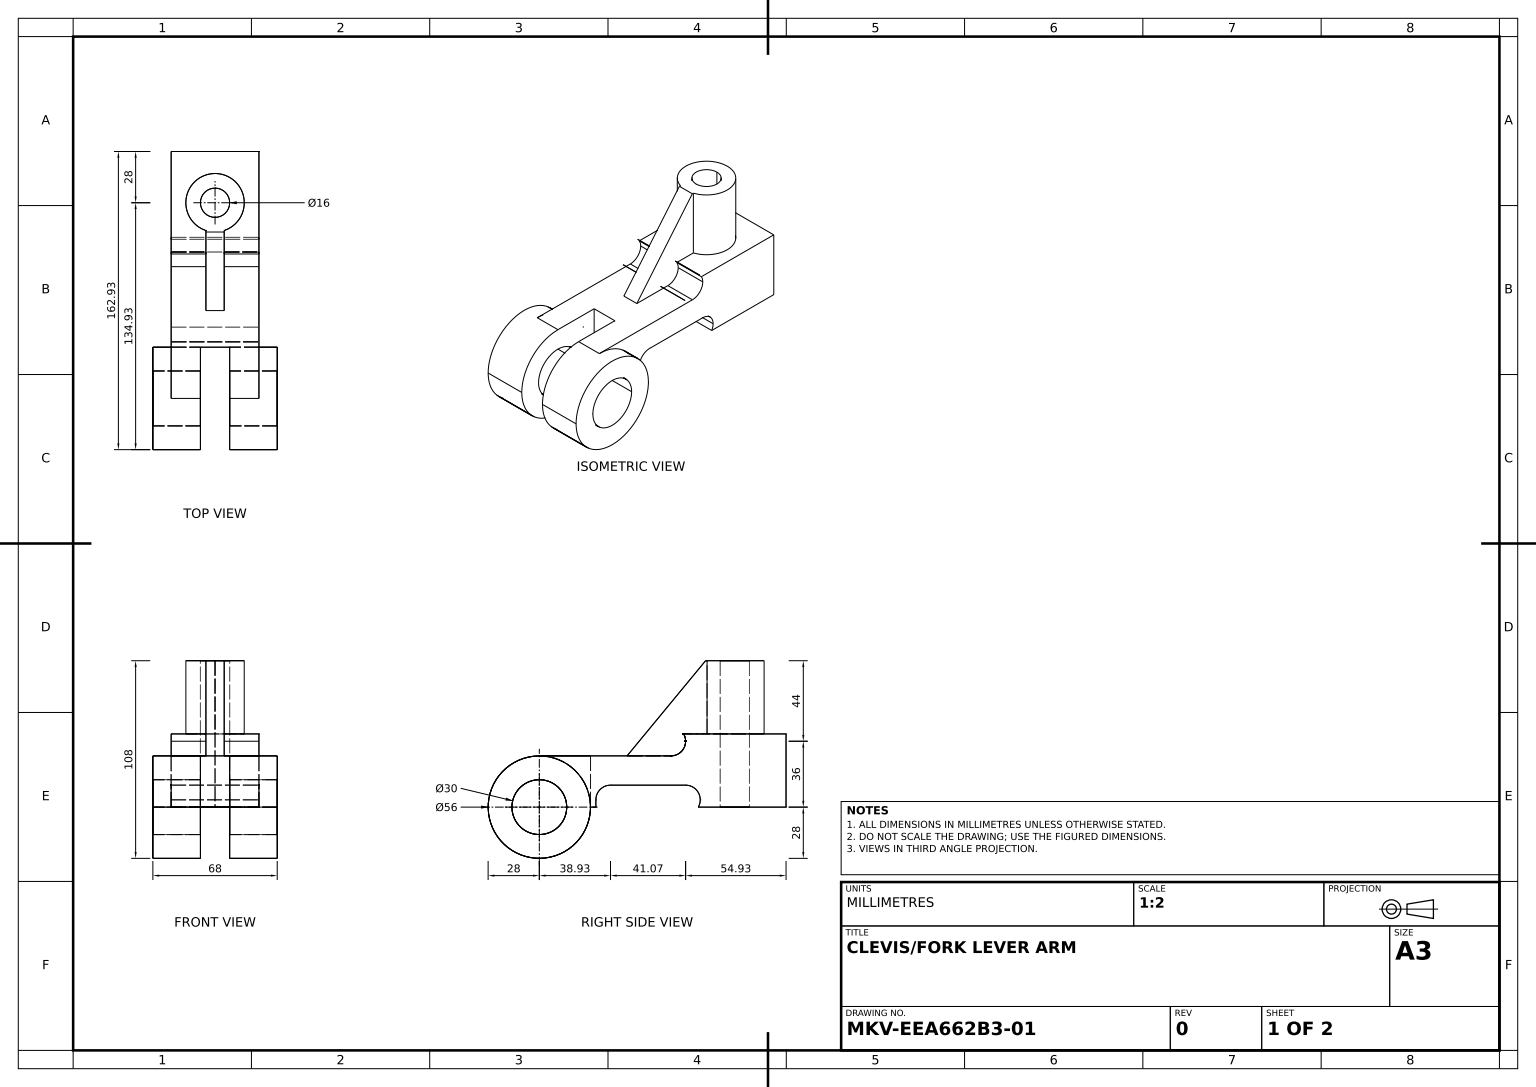
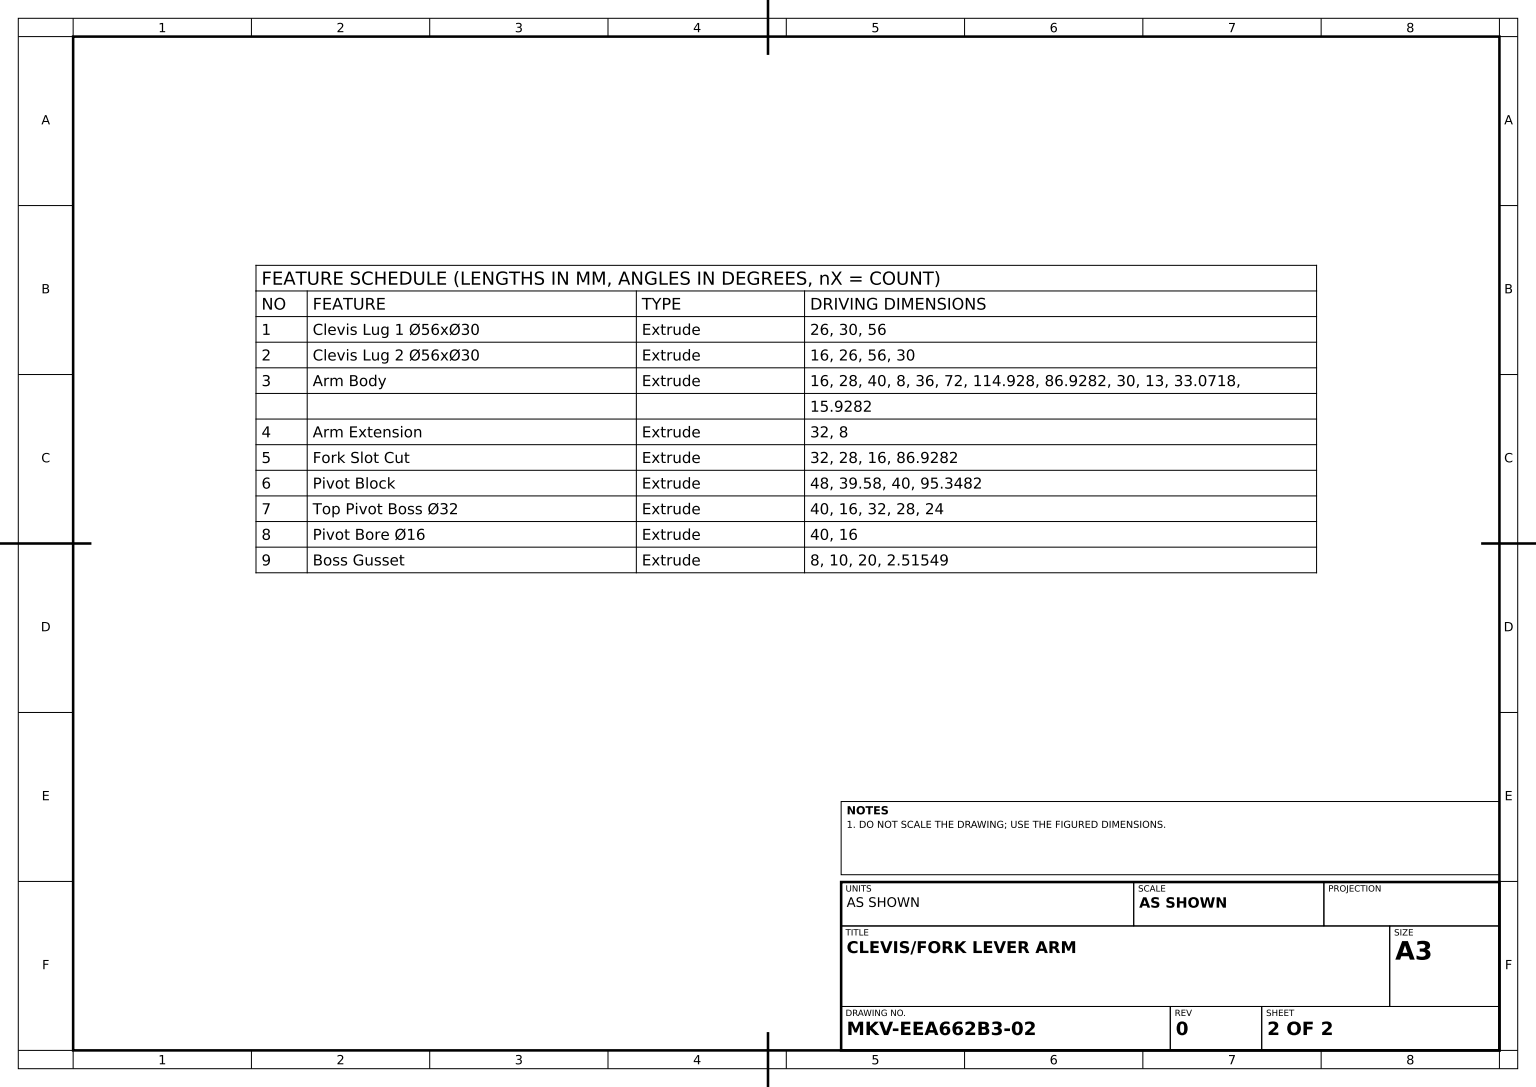
SolidWorks part; units mm, degrees
material "Plain Carbon Steel"
ref_plane "Front Plane" through (0, 0, 0) normal (0, 0, 1) x (1, 0, 0)
ref_plane "Top Plane" through (0, 0, 0) normal (0, 1, 0) x (1, 0, 0)
ref_plane "Right Plane" through (0, 0, 0) normal (1, 0, 0) x (0, 0, -1)
sketch "Clevis Lug 1 Sketch" plane through (0, 0, 0) normal (1, 0, 0) x (0, 0, -1)
  circle A0 centre (0, 0) radius 15
  circle A1 centre (0, 0) radius 28
  dimension "D1" = 30
  dimension "D2" = 56
extrude "Clevis Lug 1 Ø56xØ30" add sketch "Clevis Lug 1 Sketch" along normal blind 26
ref_plane "Lug 2 Offset Plane" through (-16, 0, 0) normal (1, 0, 0) x (0, 0, -1)
sketch "Clevis Lug 2 Sketch" plane through (-16, 0, 0) normal (1, 0, 0) x (0, 0, -1)
  circle A0 centre (0, 0) radius 15
  circle A1 centre (0, 0) radius 28
  dimension "D1" = 56
  dimension "D2" = 30
extrude "Clevis Lug 2 Ø56xØ30" add sketch "Clevis Lug 2 Sketch" against normal blind 26 separate body
sketch "Arm Profile Sketch" plane through (-16, 0, 0) normal (1, 0, 0) x (0, 0, -1)
  line L0 (0, 28) -> (72, 28)
  line L1 (114.9282, 0) -> (114.9282, 40)
  line L2 (114.9282, 40) -> (78.9282, 40)
  line L3 (114.9282, 0) -> (86.9282, 0)
  line L4 (15, 0) -> (30.9282, 0)
  line L5 (72, 12) -> (80, 12)
  line L6 (86.9282, 0) -> (30.9282, 0)
  line L7 (30.9282, 0) -> (30.9282, 4)
  line L8 (0, 28) -> (0, 15)
  line L9 (38.9282, 12) -> (72, 12)
  circle A0 centre (0, 0) radius 28 construction
  arc A1 (78.9282, 40) -> (72, 28) centre (72, 36) cw
  arc A2 (80, 12) -> (86.9282, 0) centre (80, 4) cw
  arc A3 (15, 0) -> (0, 15) centre (0, 0) ccw
  arc A4 (30.9282, 4) -> (38.9282, 12) centre (38.9282, 4) cw
  point P1 (0, 12)
  circle M11 centre (0, 0) radius 28
  dimension "D5" = 8
  dimension "D10" = 8
  dimension "D11" = 30
  dimension "D9" = 8
  dimension "D1" = 72
  dimension "D2" = 114.9282
  dimension "D3" = 28
  dimension "D4" = 40
  dimension "D6" = 36
  dimension "D7" = 28
  dimension "D8" = 86.9282
  dimension "D12" = 13
  dimension "D13" = 33.0718
  dimension "D14" = 8
  dimension "D15" = 15.9282
  dimension "D16" = 8
extrude "Arm Body" add sketch "Arm Profile Sketch" against normal blind 16 contours L7 A4 L9 L5 A2 L3 L1 L2 A1 L0 L4 M11
sketch "Arm Extension Sketch" plane through (0, 0, 0) normal (-1, 0, 0) x (0, 0, 1)
  line L0 (0, 28) -> (-72, 28)
  line L1 (-78.9282, 40) -> (-114.9282, 40)
  line L2 (-114.9282, 40) -> (-114.9282, 0)
  line L3 (-114.9282, 0) -> (-86.9282, 0)
  line L4 (-80, 12) -> (-38.9282, 12)
  line L5 (-15, 0) -> (-30.9282, 0)
  line L6 (-30.9282, 0) -> (-30.9282, 4)
  line L7 (0, 28) -> (0, 15)
  arc A0 (-72, 28) -> (-78.9282, 40) centre (-72, 36) cw
  arc A1 (-86.9282, 0) -> (-80, 12) centre (-80, 4) cw
  arc A2 (-38.9282, 12) -> (-30.9282, 4) centre (-38.9282, 4) cw
  circle A3 centre (0, 0) radius 15 construction
  arc A4 (0, 15) -> (-15, 0) centre (0, 0) ccw
  dimension "D1" = 8
extrude "Arm Extension" add sketch "Arm Extension Sketch" along normal mid plane 32
sketch "Fork Slot Sketch" plane through (0, 28, 0) normal (0, 1, 0) x (1, 0, 0)
  line L0 (-16, 0) -> (0, 0)
  line L2 (0, 0) -> (0, 28)
  line L3 (-16, 0) -> (-16, 28)
  line L4 (-16, 28) -> (0, 28)
  line L6 (-32, 114.9282) -> (16, 114.9282) construction
  dimension "D1" = 28
  dimension "D3" = 28
  dimension "D2" = 16
  dimension "D4" = 16
  dimension "D5" = 86.9282
  dimension "D6" = 16
extrude "Fork Slot Cut" cut sketch "Fork Slot Sketch" against normal blind 32
sketch "Pivot Block Sketch" plane through (16, 0, 0) normal (1, 0, 0) x (0, 0, -1)
  line L0 (95.3482, 40) -> (134.9282, 40)
  line L1 (134.9282, 40) -> (134.9282, 0)
  line L2 (134.9282, 0) -> (95.3482, 0)
  line L3 (114.9282, 0) -> (86.9282, 0) construction
  line L4 (95.3482, 0) -> (95.3482, 40)
  dimension "D1" = 39.58
  dimension "D2" = 40
  dimension "D3" = 39.58
  dimension "D4" = 95.3482
extrude "Pivot Block" add sketch "Pivot Block Sketch" against normal blind 48
sketch "Top Pivot Boss Sketch" plane through (0, 40, 0) normal (0, 1, 0) x (1, 0, 0)
  line L0 (-32, 134.9282) -> (16, 134.9282) construction
  line L1 (16, 78.9282) -> (16, 134.9282) construction
  circle A0 centre (-8, 106.9282) radius 8
  circle A1 centre (-8, 106.9282) radius 16
  dimension "D1" = 16
  dimension "D2" = 32
  dimension "D3" = 28
  dimension "D4" = 24
extrude "Top Pivot Boss Ø32" add sketch "Top Pivot Boss Sketch" along normal blind 40
sketch "Pivot Bore Sketch" plane through (0, 40, 0) normal (0, 1, 0) x (1, 0, 0)
  circle A0 centre (-8, 106.9282) radius 8
  dimension "D1" = 16
extrude "Pivot Bore Ø16" cut sketch "Pivot Bore Sketch" against normal blind 40
ref_plane "Gusset Mid Plane" through (-8, 0, 0) normal (1, 0, 0) x (0, 0, -1)
sketch "Boss Gusset Sketch" plane through (-8, 0, 0) normal (1, 0, 0) x (0, 0, -1)
  line L0 (90.9282, 80) -> (48, 28)
  line L1 (0, 28) -> (72, 28) construction
  line L2 (90.9282, 80) -> (93.4437, 80)
  line L3 (122.9282, 80) -> (90.9282, 80) construction
  line L4 (93.4437, 80) -> (93.4437, 40)
  line L5 (134.9282, 40) -> (78.9282, 40) construction
  line L6 (93.4437, 40) -> (78.9282, 40)
  line L7 (72, 28) -> (48, 28)
  arc A0 (78.9282, 40) -> (72, 28) centre (72, 36) cw
  dimension "D2" = 2.5155
  dimension "D3" = 8
  dimension "D1" = 20
extrude "Boss Gusset" add sketch "Boss Gusset Sketch" along normal mid plane 10
